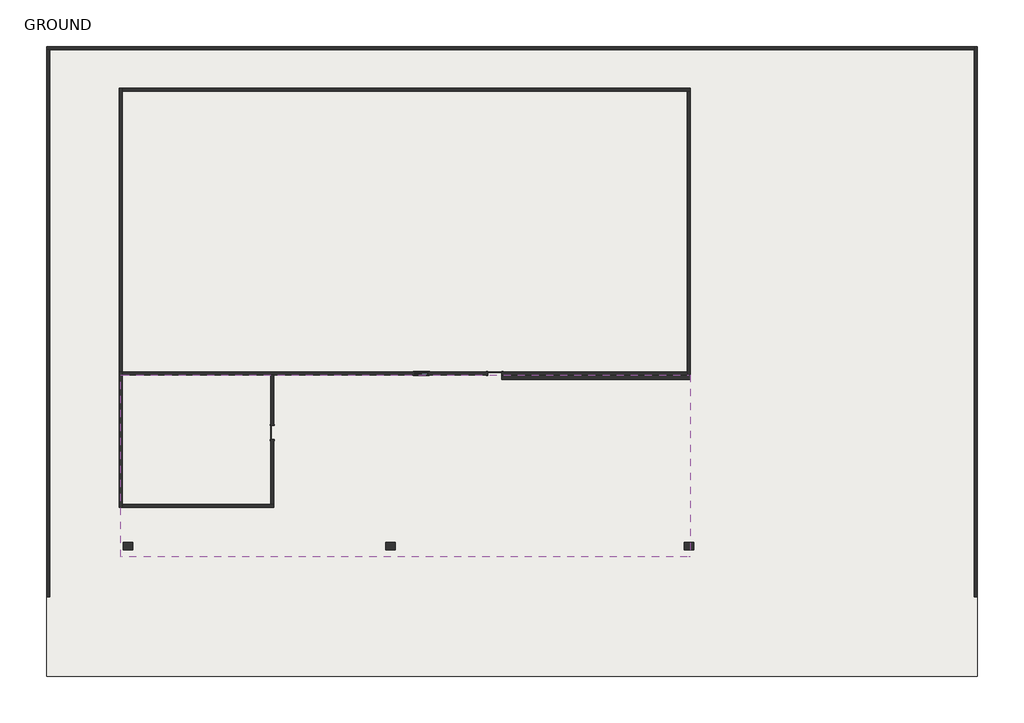
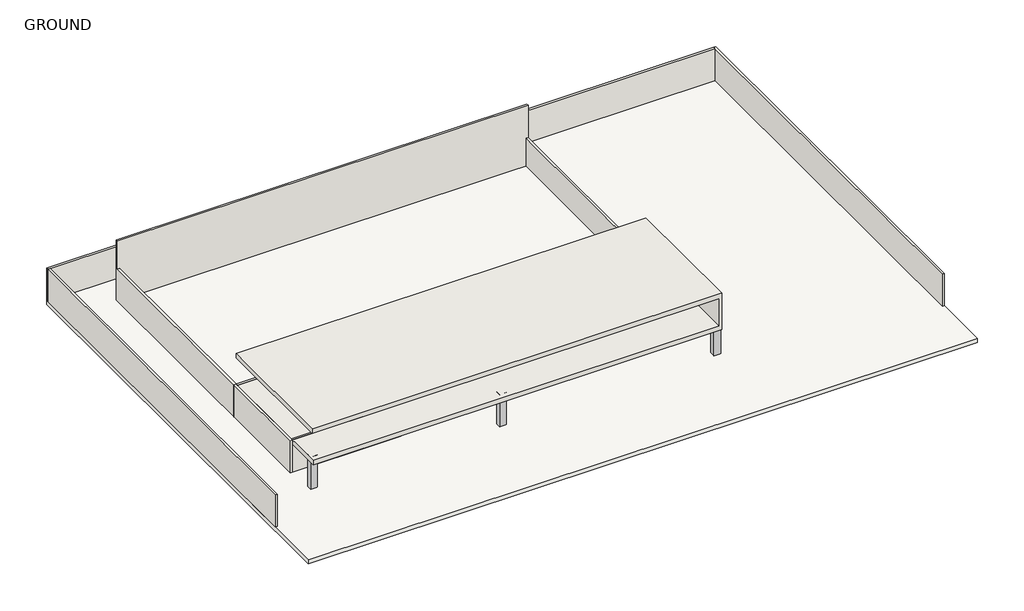
# One storey: 12 walls, 3 columns, 2 doors, 1 slab, 1 window.
"""IFC4 building model written with IfcOpenShell, lengths in millimetres."""

from ifc_helpers import new_model, si_unit, frame, origin, origin_with_axes, place, context, project, spatial, polyline, outline, extrude, faceted_brep, transform, mapped, element, save
from components import m_rectangular_column_475_x_610mm_5ff218ee, m_single_flush_0915_x_2134mm_727434cd, m_single_flush_0915_x_2134mm_6a9e8738, walls_1_walls_1_47b1a65c, walls_3_walls_3_546fd62f, window_242facca

model = new_model("IFC4")

# Units and contexts
model_context = context("Model", 3, world=origin())
ifc_project = project(units=[si_unit("LENGTHUNIT", "METRE", prefix="MILLI")], contexts=[model_context])

# Site, building, storey
site = spatial("IfcSite", under=ifc_project)
building = spatial("IfcBuilding", under=site)
storey = spatial("IfcBuildingStorey", under=building, Name="GROUND", Elevation=0.0)

# Columns
placement = place(None, origin())
m_rectangular_column_475_x_610mm_shape = m_rectangular_column_475_x_610mm_5ff218ee(model_context)
element("IfcColumn", 1, ObjectType="M_Rectangular Column : 475 x 610mm", at=placement, inside=storey, context=model_context, shape_type="MappedRepresentation", body=[
    mapped(m_rectangular_column_475_x_610mm_shape, transform((-18354.9660557, -12026.2064876, 0.0), x_axis=(1.0, 0.0, 0.0), y_axis=(0.0, 1.0, 0.0), z_axis=(0.0, 0.0, 1.0))),
])
element("IfcColumn", 2, ObjectType="M_Rectangular Column : 475 x 610mm", at=placement, inside=storey, context=model_context, shape_type="MappedRepresentation", body=[
    mapped(m_rectangular_column_475_x_610mm_shape, transform((-1438.7660557, -12026.2064876, 0.0), x_axis=(1.0, 0.0, 0.0), y_axis=(0.0, 1.0, 0.0), z_axis=(0.0, 0.0, 1.0))),
])
element("IfcColumn", 3, ObjectType="M_Rectangular Column : 475 x 610mm", at=placement, inside=storey, context=model_context, shape_type="MappedRepresentation", body=[
    mapped(m_rectangular_column_475_x_610mm_shape, transform((17763.6339443, -12026.2064876, 0.0), x_axis=(1.0, 0.0, 0.0), y_axis=(0.0, 1.0, 0.0), z_axis=(0.0, 0.0, 1.0))),
])

# Doors
m_single_flush_0915_x_2134mm_shape = m_single_flush_0915_x_2134mm_727434cd(model_context)
element("IfcDoor", 4, ObjectType="M_Single-Flush : 0915 x 2134mm", at=placement, inside=storey, context=model_context, shape_type="MappedRepresentation", body=[
    mapped(m_single_flush_0915_x_2134mm_shape, transform((-9058.7660557, -4711.0064876, 0.0), x_axis=(0.0, -1.0, 0.0), y_axis=(1.0, 0.0, 0.0), z_axis=(0.0, 0.0, 1.0))),
])
m_single_flush_0915_x_2134mm_2_shape = m_single_flush_0915_x_2134mm_6a9e8738(model_context)
element("IfcDoor", 5, ObjectType="M_Single-Flush : 0915 x 2134mm", at=placement, inside=storey, context=model_context, shape_type="MappedRepresentation", body=[
    mapped(m_single_flush_0915_x_2134mm_2_shape, transform((5266.8339443, -901.0064876, 0.0), x_axis=(1.0, 0.0, 0.0), y_axis=(0.0, 1.0, 0.0), z_axis=(0.0, 0.0, 1.0))),
])

# Slab
element("IfcSlab", 6, ObjectType="Generic Floor - 400mm", at=placement, inside=storey, context=model_context, shape_type="SweptSolid", body=[
    extrude(outline(polyline([(36349.6020876, 20162.4959969), (36349.6020876, -20408.2064876), (-23591.1979124, -20408.2064876), (-23591.1979124, 20162.4959969), (36349.6020876, 20162.4959969)])), frame((0.0, 0.0, -400.0), z_axis=(0.0, 0.0, 1.0), x_axis=(1.0, 0.0, 0.0)), (0.0, 0.0, 1.0), 400.0),
])

# Walls
element("IfcWall", 7, ObjectType="Generic - 9\"", at=placement, inside=storey, context=model_context, shape_type="Brep", body=[
    faceted_brep([(-23591.1979124, 19962.4959969, 0.0), (-23391.1979124, 19962.4959969, 0.0), (36149.6020876, 19962.4959969, 0.0), (36149.6020876, 19962.4959969, 3048.0), (-23391.1979124, 19962.4959969, 3048.0), (-23591.1979124, 19962.4959969, 3048.0), (-23591.1979124, 20162.4959969, 0.0), (-23591.1979124, 20162.4959969, 3048.0), (36149.6020876, 20162.4959969, 3048.0), (36149.6020876, 20162.4959969, 0.0)], [[[0, 1, 2, 3, 4, 5]], [[6, 7, 8, 9]], [[2, 1, 0, 6, 9]], [[5, 4, 3, 8, 7]], [[0, 5, 7, 6]], [[3, 2, 9, 8]]]),
])
element("IfcWall", 8, ObjectType="Generic - 9\"", at=placement, inside=storey, context=model_context, shape_type="SweptSolid", body=[
    extrude(outline(polyline([(-23391.1979124, 19962.4959969), (-23391.1979124, -15294.3040031), (-23591.1979124, -15294.3040031), (-23591.1979124, 19962.4959969), (-23391.1979124, 19962.4959969)])), origin_with_axes(), (0.0, 0.0, 1.0), 3048.0),
])
element("IfcWall", 9, ObjectType="Generic - 9\"", at=placement, inside=storey, context=model_context, shape_type="Brep", body=[
    faceted_brep([(36149.6020876, 20162.4959969, 0.0), (36149.6020876, 19962.4959969, 0.0), (36149.6020876, -15294.3040031, 0.0), (36149.6020876, -15294.3040031, 3048.0), (36149.6020876, 19962.4959969, 3048.0), (36149.6020876, 20162.4959969, 3048.0), (36349.6020876, 20162.4959969, 0.0), (36349.6020876, 20162.4959969, 3048.0), (36349.6020876, -15294.3040031, 3048.0), (36349.6020876, -15294.3040031, 0.0)], [[[0, 1, 2, 3, 4, 5]], [[6, 7, 8, 9]], [[2, 1, 0, 6, 9]], [[3, 2, 9, 8]], [[5, 4, 3, 8, 7]], [[0, 5, 7, 6]]]),
])
element("IfcWall", 10, ObjectType="Generic - 9\"", at=placement, inside=storey, context=model_context, shape_type="Brep", body=[
    faceted_brep([(-18712.3660557, -9535.4064876, 0.0), (-18712.3660557, -9335.4064876, 0.0), (-18712.3660557, -1001.0064876, 0.0), (-18712.3660557, -801.0064876, 0.0), (-18712.3660557, -801.0064876, 3048.0), (-18712.3660557, -1001.0064876, 3048.0), (-18712.3660557, -9335.4064876, 3048.0), (-18712.3660557, -9535.4064876, 3048.0), (-18912.3660557, -9535.4064876, 0.0), (-18912.3660557, -9535.4064876, 3048.0), (-18912.3660557, -801.0064876, 3048.0), (-18912.3660557, -801.0064876, 0.0)], [[[0, 1, 2, 3, 4, 5, 6, 7]], [[8, 9, 10, 11]], [[3, 2, 1, 0, 8, 11]], [[7, 6, 5, 4, 10, 9]], [[0, 7, 9, 8]], [[4, 3, 11, 10]]]),
])
element("IfcWall", 11, ObjectType="Generic - 9\"", at=placement, inside=storey, context=model_context, shape_type="Brep", body=[
    faceted_brep([(-8958.7660557, -9335.4064876, 0.0), (-9158.7660557, -9335.4064876, 0.0), (-18712.3660557, -9335.4064876, 0.0), (-18712.3660557, -9335.4064876, 3048.0), (-9158.7660557, -9335.4064876, 3048.0), (-8958.7660557, -9335.4064876, 3048.0), (-8958.7660557, -9535.4064876, 0.0), (-8958.7660557, -9535.4064876, 3048.0), (-18712.3660557, -9535.4064876, 3048.0), (-18712.3660557, -9535.4064876, 0.0)], [[[0, 1, 2, 3, 4, 5]], [[6, 7, 8, 9]], [[2, 1, 0, 6, 9]], [[5, 4, 3, 8, 7]], [[0, 5, 7, 6]], [[3, 2, 9, 8]]]),
])
element("IfcWall", 12, ObjectType="Generic - 9\"", at=placement, inside=storey, context=model_context, shape_type="SweptSolid", body=[
    extrude(outline(polyline([(-5168.5064876, 2134.0), (-5168.5064876, 0.0), (-9335.4064876, 0.0), (-9335.4064876, 3048.0), (-1001.0064876, 3048.0), (-1001.0064876, 0.0), (-4253.5064876, 0.0), (-4253.5064876, 2134.0), (-5168.5064876, 2134.0)])), frame((-9158.7660557, 0.0, 0.0), z_axis=(1.0, 0.0, 0.0), x_axis=(0.0, 1.0, 0.0)), (0.0, 0.0, 1.0), 200.0),
])
element("IfcWall", 13, ObjectType="Generic - 9\"", at=placement, inside=storey, context=model_context, shape_type="Brep", body=[
    faceted_brep([(5724.3339443, -1001.0064876, 2134.0), (5724.3339443, -1001.0064876, 0.0), (17663.6339443, -1001.0064876, 0.0), (17663.6339443, -1001.0064876, 2648.0), (17663.6339443, -1001.0064876, 3048.0), (-8958.7660557, -1001.0064876, 3048.0), (-9158.7660557, -1001.0064876, 3048.0), (-18712.3660557, -1001.0064876, 3048.0), (-18712.3660557, -1001.0064876, 0.0), (-9158.7660557, -1001.0064876, 0.0), (-8958.7660557, -1001.0064876, 0.0), (4809.3339443, -1001.0064876, 0.0), (4809.3339443, -1001.0064876, 2134.0), (999.6339443, -1001.0064876, 2133.6), (999.6339443, -1001.0064876, 914.4), (85.2339443, -1001.0064876, 914.4), (85.2339443, -1001.0064876, 2133.6), (17663.6339443, -801.0064876, 0.0), (5724.3339443, -801.0064876, 0.0), (5724.3339443, -801.0064876, 2134.0), (4809.3339443, -801.0064876, 2134.0), (4809.3339443, -801.0064876, 0.0), (-18712.3660557, -801.0064876, 0.0), (-18712.3660557, -801.0064876, 3048.0), (17663.6339443, -801.0064876, 3048.0), (999.6339443, -801.0064876, 2133.6), (85.2339443, -801.0064876, 2133.6), (85.2339443, -801.0064876, 914.4), (999.6339443, -801.0064876, 914.4)], [[[0, 1, 2, 3, 4, 5, 6, 7, 8, 9, 10, 11, 12], [13, 14, 15, 16]], [[17, 18, 19, 20, 21, 22, 23, 24], [25, 26, 27, 28]], [[2, 1, 18, 17]], [[11, 10, 9, 8, 22, 21]], [[7, 6, 5, 4, 24, 23]], [[4, 3, 2, 17, 24]], [[8, 7, 23, 22]], [[19, 18, 1, 0]], [[20, 19, 0, 12]], [[21, 20, 12, 11]], [[14, 13, 25, 28]], [[15, 14, 28, 27]], [[16, 15, 27, 26]], [[13, 16, 26, 25]]]),
])
element("IfcWall", 14, ObjectType="Generic - 9\"", at=placement, inside=storey, context=model_context, shape_type="Brep", body=[
    faceted_brep([(-18912.3660557, 17486.9935124, 0.0), (-18912.3660557, -801.0064876, 0.0), (-18912.3660557, -801.0064876, 3048.0), (-18912.3660557, 17286.9935124, 3048.0), (-18912.3660557, 17486.9935124, 3048.0), (-18712.3660557, 17486.9935124, 0.0), (-18712.3660557, 17486.9935124, 3048.0), (-18712.3660557, 17286.9935124, 3048.0), (-18712.3660557, -801.0064876, 3048.0), (-18712.3660557, -801.0064876, 0.0), (-18712.3660557, 17286.9935124, 0.0)], [[[0, 1, 2, 3, 4]], [[5, 6, 7, 8, 9, 10]], [[1, 0, 5, 10, 9]], [[4, 3, 2, 8, 7, 6]], [[0, 4, 6, 5]], [[2, 1, 9, 8]]]),
])
element("IfcWall", 15, ObjectType="Generic - 9\"", at=placement, inside=storey, context=model_context, shape_type="Brep", body=[
    faceted_brep([(17863.6339443, 17486.9935124, 5700.0), (17863.6339443, 17486.9935124, 0.0), (-18712.3660557, 17486.9935124, 0.0), (-18712.3660557, 17486.9935124, 3048.0), (-18912.3660557, 17486.9935124, 3048.0), (-18912.3660557, 17486.9935124, 5700.0), (17863.6339443, 17286.9935124, 0.0), (17863.6339443, 17286.9935124, 2648.0), (17863.6339443, 17286.9935124, 3048.0), (17863.6339443, 17286.9935124, 5700.0), (-18912.3660557, 17286.9935124, 5700.0), (-18912.3660557, 17286.9935124, 3048.0), (-18712.3660557, 17286.9935124, 3048.0), (-18712.3660557, 17286.9935124, 0.0), (17663.6339443, 17286.9935124, 0.0)], [[[0, 1, 2, 3, 4, 5]], [[6, 7, 8, 9, 10, 11, 12, 13, 14]], [[2, 1, 6, 14, 13]], [[0, 5, 10, 9]], [[0, 9, 8, 7, 6, 1]], [[11, 4, 3, 12]], [[3, 2, 13, 12]], [[5, 4, 11, 10]]]),
])
element("IfcWall", 16, ObjectType="Generic - 9\"", at=placement, inside=storey, context=model_context, shape_type="Brep", body=[
    faceted_brep([(17863.6339443, -1001.0064876, 0.0), (17863.6339443, 17286.9935124, 0.0), (17863.6339443, 17286.9935124, 2648.0), (17863.6339443, -1001.0064876, 2648.0), (17663.6339443, -1001.0064876, 0.0), (17663.6339443, -1001.0064876, 2648.0), (17663.6339443, 17286.9935124, 2648.0), (17663.6339443, 17286.9935124, 0.0), (17663.6339443, -801.0064876, 0.0)], [[[0, 1, 2, 3]], [[4, 5, 6, 7, 8]], [[1, 0, 4, 8, 7]], [[3, 2, 6, 5]], [[0, 3, 5, 4]], [[2, 1, 7, 6]]]),
])
walls_1_walls_1_shape = walls_1_walls_1_47b1a65c(model_context)
element("IfcWall", 17, ObjectType="Walls 1 : Walls 1", at=placement, inside=storey, context=model_context, shape_type="MappedRepresentation", body=[
    mapped(walls_1_walls_1_shape, transform((0.0, 0.0, 0.0), x_axis=(1.0, 0.0, 0.0), y_axis=(0.0, 1.0, 0.0), z_axis=(0.0, 0.0, 1.0))),
])
walls_3_walls_3_shape = walls_3_walls_3_546fd62f(model_context)
element("IfcWall", 18, ObjectType="Walls 3 : Walls 3", at=placement, inside=storey, context=model_context, shape_type="MappedRepresentation", body=[
    mapped(walls_3_walls_3_shape, transform((0.0, 0.0, 0.0), x_axis=(1.0, 0.0, 0.0), y_axis=(0.0, 1.0, 0.0), z_axis=(0.0, 0.0, 1.0))),
])

# Window
window_shape = window_242facca(model_context)
element("IfcWindow", 19, ObjectType="Slider with Trim : 36\" x 48\"", at=placement, inside=storey, context=model_context, shape_type="MappedRepresentation", body=[
    mapped(window_shape, transform((542.4339443, -901.0064876, 0.0), x_axis=(1.0, 0.0, 0.0), y_axis=(0.0, 1.0, 0.0), z_axis=(0.0, 0.0, 1.0))),
])

save(model, "model.ifc")

# Revit data of these elements
# Type "M_Rectangular Column : 475 x 610mm"
#   Depth = 475 mm
#   Offset Base = 0 mm
#   Offset Top = 0 mm
#   Width = 610 mm
#   Material = none
# Type "M_Single-Flush : 0915 x 2134mm"
#   Type Mark = "15"
#   Thickness = 51 mm
#   Height = 2134 mm
#   Trim Projection Ext = 25 mm
#   Trim Projection Int = 25 mm
#   Trim Width = 76 mm
#   Width = 915 mm
#   Door Material = Door - Panel
#   Frame Material = Door - Frame
#   Function = (empty or 0)
#   Wall Closure = (empty or 0)
# Type "Generic Floor - 400mm"
#   Function = 0
#   Layers, outside or top first: 400 mm no material (function 1)
# Type "Generic - 9\""
#   Layers, outside or top first: 200 mm no material (function 1)
# Type "Slider with Trim : 36\" x 48\""
#   Type Mark = "19"
#   Construction Type Id = "GSP4R"
#   Assembly Code = "B2020100"
#   Analytic Construction = "1/8 in Pilkington single glazing"
#   Visual Light Transmittance = 0.9
#   Solar Heat Gain Coefficient = 0.78
#   Heat Transfer Coefficient (U) = 3.6886 W/(m²·K)
#   Height = 1219.2 mm
#   Default Sill Height = 914.4 mm
#   Trim Projection - Ext. = 19.05 mm
#   Trim Projection - Int. = 19.05 mm
#   Trim Width - Exterior = 88.9 mm
#   Trim Width - Interior = 88.9 mm
#   Width = 914.4 mm
#   Window Inset = 19.05 mm
#   Define Thermal Properties by = 1
#   Glass Pane Material = Glass
#   Sash Material = Sash
#   Trim Exterior Material = Trim
#   Trim Interior Material = Trim
#   Wall Closure = (empty or 0)
# Elements 1, 2, 3 (IfcColumn, "M_Rectangular Column : 475 x 610mm")
#   Phase Created = New Construction
# Elements 4, 5 (IfcDoor, "M_Single-Flush : 0915 x 2134mm")
#   Phase Created = New Construction
#   Materials on its faces: "Door - Frame", "Door - Panel"
# Element 6 (IfcSlab, "Generic Floor - 400mm")
#   Height Offset From Level = 0 mm
#   Phase Created = New Construction
#   Materials on its faces: "Default Roof"
# Elements 7, 8, 9, 10, 11, 12, 13, 14 (IfcWall, "Generic - 9\"")
#   Top Offset = 0 mm
#   Base Offset = 0 mm
#   Unconnected Height = 3048 mm
#   wall height = 3048 mm
#   Phase Created = New Construction
#   Base Constraint = GROUND
#   Materials on its faces: "Default Wall"
# Element 15 (IfcWall, "Generic - 9\"")
#   Top Offset = 0 mm
#   Base Offset = 0 mm
#   Unconnected Height = 5700 mm
#   wall height = 5700 mm
#   Phase Created = New Construction
#   Base Constraint = GROUND
#   Materials on its faces: "Default Wall"
# Element 16 (IfcWall, "Generic - 9\"")
#   Top Offset = 0 mm
#   Base Offset = 0 mm
#   Unconnected Height = 2648 mm
#   wall height = 2648 mm
#   Phase Created = New Construction
#   Base Constraint = GROUND
#   Materials on its faces: "Default Wall"
# Element 17 (IfcWall, "Walls 1 : Walls 1")
#   Phase Created = New Construction
#   Materials on its faces: "Default Wall"
# Element 18 (IfcWall, "Walls 3 : Walls 3")
#   Phase Created = New Construction
#   Materials on its faces: "Default Wall"
# Element 19 (IfcWindow, "Slider with Trim : 36\" x 48\"")
#   Mark = "8"
#   Phase Created = New Construction
#   Materials on its faces: "Sash", "Trim", "Glass"
# Materials
#   "Door - Panel": class "Wood", colour RGB 114 82 51, transparency 0
#   "Door - Frame": colour RGB 153 76 43, transparency 0
#   "Glass": class "Glass", colour RGB 218 227 224, transparency 0.85, Description = "Soda Lime Glass", Cost = 0
#   "Sash": class "Wood", colour RGB 136 99 55, transparency 0
#   "Trim": class "Wood", colour RGB 224 178 126, transparency 0
#   "Default Roof": colour RGB 80 80 80, transparency 0
#   "Default Wall": colour RGB 80 80 80, transparency 0
